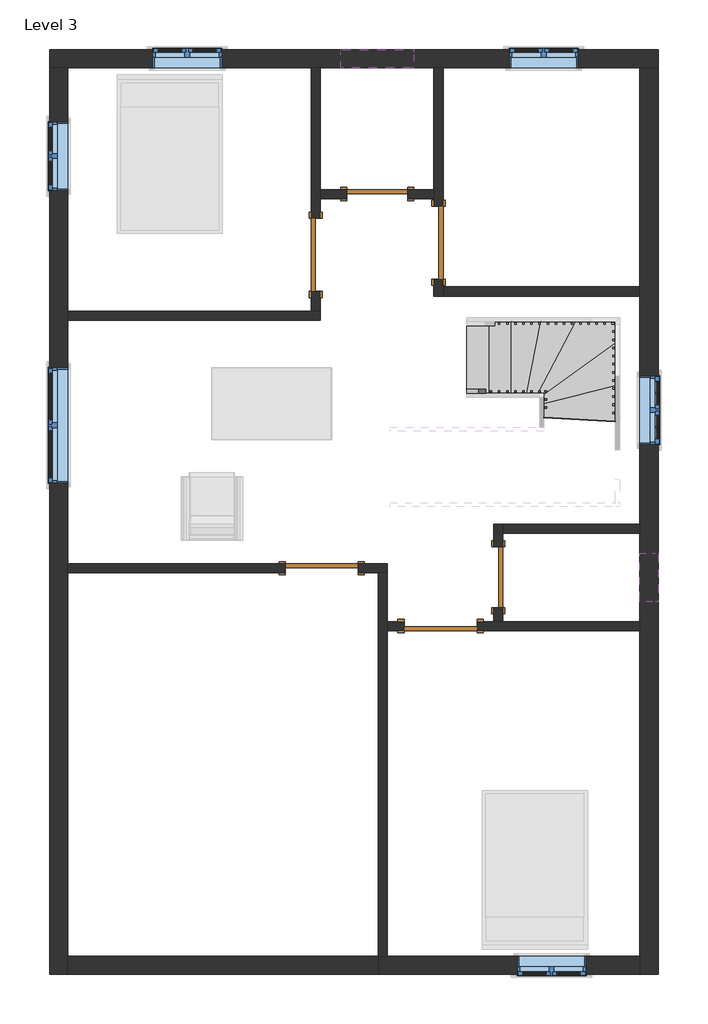
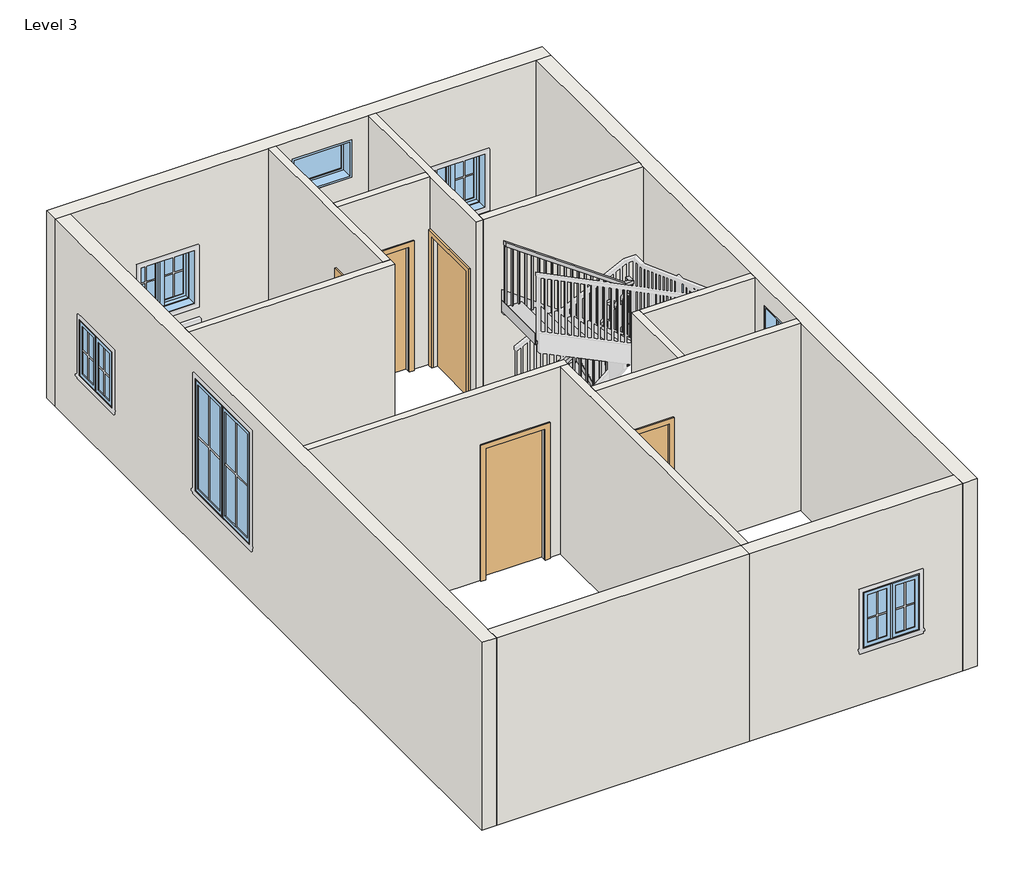
# One storey, part 1 of 2: 15 walls, 8 windows, 6 doors, 1 railing, 1 stair flight.
"""IFC4 building model written with IfcOpenShell, lengths in millimetres."""

from ifc_helpers import new_model, si_unit, frame, origin, place, context, project, spatial, polyline, outline, extrude, faceted_brep, transform, mapped, element, save
from components import door_d8f5dbb5, door_f2b275c1, door_e5f9f3c4, door_305aa2a5, stair_flight_546a6d32, window_80340324, window_bb95b1c9, window_339605e1, window_9ac97e1a

model = new_model("IFC4")

# Units and contexts
model_context = context("Model", 3, world=origin())
ifc_project = project(units=[si_unit("LENGTHUNIT", "METRE", prefix="MILLI")], contexts=[model_context])

# Site, building, storey
site = spatial("IfcSite", under=ifc_project)
building = spatial("IfcBuilding", under=site)
storey = spatial("IfcBuildingStorey", under=building, Name="Level 3", Elevation=3200.4)

# Doors
placement = place(None, origin())
door_shape = door_d8f5dbb5(model_context)
element("IfcDoor", 1, ObjectType="Single-Flush : 30\" x 80\"", at=placement, inside=storey, context=model_context, shape_type="MappedRepresentation", body=[
    mapped(door_shape, transform((-963.1415084, 4519.6435985, 3200.4), x_axis=(1.0, 0.0, 0.0), y_axis=(0.0, 1.0, 0.0), z_axis=(0.0, 0.0, 1.0))),
])
door_2_shape = door_f2b275c1(model_context)
element("IfcDoor", 2, ObjectType="Single-Flush : 30\" x 80\"", at=placement, inside=storey, context=model_context, shape_type="MappedRepresentation", body=[
    mapped(door_2_shape, transform((554.5084916, -280.9564015, 3200.4), x_axis=(0.0, 1.0, 0.0), y_axis=(-1.0, 0.0, 0.0), z_axis=(0.0, 0.0, 1.0))),
])
door_3_shape = door_e5f9f3c4(model_context)
element("IfcDoor", 3, ObjectType="Single-Flush : 36\" x 84\"", at=placement, inside=storey, context=model_context, shape_type="MappedRepresentation", body=[
    mapped(door_3_shape, transform((-194.7915084, 3910.0435985, 3200.4), x_axis=(0.0, -1.0, 0.0), y_axis=(1.0, 0.0, 0.0), z_axis=(0.0, 0.0, 1.0))),
])
element("IfcDoor", 4, ObjectType="Single-Flush : 36\" x 84\"", at=placement, inside=storey, context=model_context, shape_type="MappedRepresentation", body=[
    mapped(door_3_shape, transform((-1655.2915084, -166.6564015, 3200.4), x_axis=(1.0, 0.0, 0.0), y_axis=(0.0, 1.0, 0.0), z_axis=(0.0, 0.0, 1.0))),
])
element("IfcDoor", 5, ObjectType="Single-Flush : 36\" x 84\"", at=placement, inside=storey, context=model_context, shape_type="MappedRepresentation", body=[
    mapped(door_3_shape, transform((-169.3915084, -890.5564015, 3200.4), x_axis=(-1.0, 0.0, 0.0), y_axis=(0.0, -1.0, 0.0), z_axis=(0.0, 0.0, 1.0))),
])
door_4_shape = door_305aa2a5(model_context)
element("IfcDoor", 6, ObjectType="Single-Flush : 36\" x 84\"", at=placement, inside=storey, context=model_context, shape_type="MappedRepresentation", body=[
    mapped(door_4_shape, transform((-1731.4915084, 3757.6435985, 3200.4), x_axis=(0.0, -1.0, 0.0), y_axis=(1.0, 0.0, 0.0), z_axis=(0.0, 0.0, 1.0))),
])

# Railing
element("IfcRailing", 7, ObjectType="Handrail - Rectangular", at=placement, inside=storey, context=model_context, shape_type="SolidModel", body=[
    faceted_brep([(158.6923968, 2074.8935985, 4284.1333333), (158.6923968, 2074.8935985, 4220.4053174), (158.6923968, 2024.0935985, 4220.4053174), (158.6923968, 2024.0935985, 4284.1333333), (1047.1901835, 2074.8935985, 4957.132376), (1097.9901835, 2074.8935985, 4931.8831856), (1097.9901835, 2024.0935985, 4931.8831856), (1047.1901835, 2024.0935985, 4957.132376), (1047.1901835, 2074.8935985, 5211.4303182), (1097.9901835, 2074.8935985, 5160.6303182), (1097.9901835, 2024.0935985, 5160.6303182), (1047.1901835, 2024.0935985, 5211.4303182), (1174.1901835, 2074.8935985, 5211.4303182), (1174.1901835, 2074.8935985, 5160.6303182), (1123.3901835, 2024.0935985, 5160.6303182), (1123.3901835, 2024.0935985, 5211.4303182), (1174.1901835, 1947.8935985, 5211.4303182), (1174.1901835, 1922.7437783, 5160.6303182), (1123.3901835, 1922.7437783, 5160.6303182), (1123.3901835, 1947.8935985, 5211.4303182), (1174.1901835, 1627.4476133, 5631.73697), (1174.1901835, 1576.6476133, 5614.5805221), (1123.3901835, 1576.6476133, 5614.5805221), (1123.3901835, 1627.4476133, 5631.73697), (1174.1901835, 1627.4476133, 5852.9821577), (1174.1901835, 1576.6476133, 5802.1821577), (1123.3901835, 1576.6476133, 5802.1821577), (1123.3901835, 1627.4476133, 5852.9821577), (1174.1901835, 1500.4476133, 5852.9821577), (1174.1901835, 1500.4476133, 5802.1821577), (1123.3901835, 1551.2476133, 5802.1821577), (1123.3901835, 1551.2476133, 5852.9821577), (1047.1901835, 1500.4476133, 5852.9821577), (1030.9951821, 1500.4476133, 5802.1821577), (1030.9951821, 1551.2476133, 5802.1821577), (1047.1901835, 1551.2476133, 5852.9821577), (-798.3242294, 1500.4476133, 7162.8), (-798.3242294, 1551.2476133, 7162.8), (-798.3242294, 1551.2476133, 7100.5059138), (-798.3242294, 1500.4476133, 7100.5059138)], [[[0, 1, 2, 3]], [[1, 0, 4, 5]], [[2, 1, 5, 6]], [[3, 2, 6, 7]], [[0, 3, 7, 4]], [[5, 4, 8, 9]], [[6, 5, 9, 10]], [[7, 6, 10, 11]], [[4, 7, 11, 8]], [[9, 8, 12, 13]], [[10, 9, 13, 14]], [[11, 10, 14, 15]], [[8, 11, 15, 12]], [[13, 12, 16, 17]], [[14, 13, 17, 18]], [[15, 14, 18, 19]], [[12, 15, 19, 16]], [[17, 16, 20, 21]], [[18, 17, 21, 22]], [[19, 18, 22, 23]], [[16, 19, 23, 20]], [[21, 20, 24, 25]], [[22, 21, 25, 26]], [[23, 22, 26, 27]], [[20, 23, 27, 24]], [[25, 24, 28, 29]], [[26, 25, 29, 30]], [[27, 26, 30, 31]], [[24, 27, 31, 28]], [[29, 28, 32, 33]], [[30, 29, 33, 34]], [[31, 30, 34, 35]], [[28, 31, 35, 32]], [[36, 37, 38, 39]], [[33, 32, 36, 39]], [[34, 33, 39, 38]], [[35, 34, 38, 37]], [[32, 35, 37, 36]]]),
    extrude(outline(polyline([(7081.8830025, -772.0848165), (7095.4033683, -791.1348165), (6079.0666667, -791.1348165), (6079.0666667, -772.0848165), (7081.8830025, -772.0848165)])), frame((0.0, 1516.3226133, 0.0), z_axis=(0.0, 1.0, 0.0), x_axis=(0.0, 0.0, 1.0)), (0.0, 0.0, 1.0), 19.05),
    extrude(outline(polyline([(7009.7743851, -670.4848165), (7023.2947509, -689.5348165), (6079.0666667, -689.5348165), (6079.0666667, -670.4848165), (7009.7743851, -670.4848165)])), frame((0.0, 1516.3226133, 0.0), z_axis=(0.0, 1.0, 0.0), x_axis=(0.0, 0.0, 1.0)), (0.0, 0.0, 1.0), 19.05),
    extrude(outline(polyline([(6937.6657677, -568.8848165), (6951.1861334, -587.9348165), (6079.0666667, -587.9348165), (6079.0666667, -568.8848165), (6937.6657677, -568.8848165)])), frame((0.0, 1516.3226133, 0.0), z_axis=(0.0, 1.0, 0.0), x_axis=(0.0, 0.0, 1.0)), (0.0, 0.0, 1.0), 19.05),
    extrude(outline(polyline([(6865.5571502, -467.2848165), (6879.077516, -486.3348165), (5909.7333333, -486.3348165), (5909.7333333, -467.2848165), (6865.5571502, -467.2848165)])), frame((0.0, 1516.3226133, 0.0), z_axis=(0.0, 1.0, 0.0), x_axis=(0.0, 0.0, 1.0)), (0.0, 0.0, 1.0), 19.05),
    extrude(outline(polyline([(6793.4485328, -365.6848165), (6806.9688986, -384.7348165), (5909.7333333, -384.7348165), (5909.7333333, -365.6848165), (6793.4485328, -365.6848165)])), frame((0.0, 1516.3226133, 0.0), z_axis=(0.0, 1.0, 0.0), x_axis=(0.0, 0.0, 1.0)), (0.0, 0.0, 1.0), 19.05),
    extrude(outline(polyline([(6721.3399154, -264.0848165), (6734.8602811, -283.1348165), (5909.7333333, -283.1348165), (5909.7333333, -264.0848165), (6721.3399154, -264.0848165)])), frame((0.0, 1516.3226133, 0.0), z_axis=(0.0, 1.0, 0.0), x_axis=(0.0, 0.0, 1.0)), (0.0, 0.0, 1.0), 19.05),
    extrude(outline(polyline([(6649.2312979, -162.4848165), (6662.7516637, -181.5348165), (5740.4, -181.5348165), (5740.4, -162.4848165), (6649.2312979, -162.4848165)])), frame((0.0, 1516.3226133, 0.0), z_axis=(0.0, 1.0, 0.0), x_axis=(0.0, 0.0, 1.0)), (0.0, 0.0, 1.0), 19.05),
    extrude(outline(polyline([(6577.1226805, -60.8848165), (6590.6430462, -79.9348165), (5740.4, -79.9348165), (5740.4, -60.8848165), (6577.1226805, -60.8848165)])), frame((0.0, 1516.3226133, 0.0), z_axis=(0.0, 1.0, 0.0), x_axis=(0.0, 0.0, 1.0)), (0.0, 0.0, 1.0), 19.05),
    extrude(outline(polyline([(6505.014063, 40.7151835), (6518.5344288, 21.6651835), (5571.0666667, 21.6651835), (5571.0666667, 40.7151835), (6505.014063, 40.7151835)])), frame((0.0, 1516.3226133, 0.0), z_axis=(0.0, 1.0, 0.0), x_axis=(0.0, 0.0, 1.0)), (0.0, 0.0, 1.0), 19.05),
    extrude(outline(polyline([(6432.9054456, 142.3151835), (6446.4258114, 123.2651835), (5571.0666667, 123.2651835), (5571.0666667, 142.3151835), (6432.9054456, 142.3151835)])), frame((0.0, 1516.3226133, 0.0), z_axis=(0.0, 1.0, 0.0), x_axis=(0.0, 0.0, 1.0)), (0.0, 0.0, 1.0), 19.05),
    extrude(outline(polyline([(6360.7968282, 243.9151835), (6374.3171939, 224.8651835), (5571.0666667, 224.8651835), (5571.0666667, 243.9151835), (6360.7968282, 243.9151835)])), frame((0.0, 1516.3226133, 0.0), z_axis=(0.0, 1.0, 0.0), x_axis=(0.0, 0.0, 1.0)), (0.0, 0.0, 1.0), 19.05),
    extrude(outline(polyline([(6288.6882107, 345.5151835), (6302.2085765, 326.4651835), (5401.7333333, 326.4651835), (5401.7333333, 345.5151835), (6288.6882107, 345.5151835)])), frame((0.0, 1516.3226133, 0.0), z_axis=(0.0, 1.0, 0.0), x_axis=(0.0, 0.0, 1.0)), (0.0, 0.0, 1.0), 19.05),
    extrude(outline(polyline([(6216.5795933, 447.1151835), (6230.0999591, 428.0651835), (5401.7333333, 428.0651835), (5401.7333333, 447.1151835), (6216.5795933, 447.1151835)])), frame((0.0, 1516.3226133, 0.0), z_axis=(0.0, 1.0, 0.0), x_axis=(0.0, 0.0, 1.0)), (0.0, 0.0, 1.0), 19.05),
    extrude(outline(polyline([(6144.4709758, 548.7151835), (6157.9913416, 529.6651835), (5232.4, 529.6651835), (5232.4, 548.7151835), (6144.4709758, 548.7151835)])), frame((0.0, 1516.3226133, 0.0), z_axis=(0.0, 1.0, 0.0), x_axis=(0.0, 0.0, 1.0)), (0.0, 0.0, 1.0), 19.05),
    extrude(outline(polyline([(6072.3623584, 650.3151835), (6085.8827242, 631.2651835), (5232.4, 631.2651835), (5232.4, 650.3151835), (6072.3623584, 650.3151835)])), frame((0.0, 1516.3226133, 0.0), z_axis=(0.0, 1.0, 0.0), x_axis=(0.0, 0.0, 1.0)), (0.0, 0.0, 1.0), 19.05),
    extrude(outline(polyline([(6000.253741, 751.9151835), (6013.7741067, 732.8651835), (5232.4, 732.8651835), (5232.4, 751.9151835), (6000.253741, 751.9151835)])), frame((0.0, 1516.3226133, 0.0), z_axis=(0.0, 1.0, 0.0), x_axis=(0.0, 0.0, 1.0)), (0.0, 0.0, 1.0), 19.05),
    extrude(outline(polyline([(5928.1451235, 853.5151835), (5941.6654893, 834.4651835), (5063.0666667, 834.4651835), (5063.0666667, 853.5151835), (5928.1451235, 853.5151835)])), frame((0.0, 1516.3226133, 0.0), z_axis=(0.0, 1.0, 0.0), x_axis=(0.0, 0.0, 1.0)), (0.0, 0.0, 1.0), 19.05),
    extrude(outline(polyline([(5856.0365061, 955.1151835), (5869.5568719, 936.0651835), (5063.0666667, 936.0651835), (5063.0666667, 955.1151835), (5856.0365061, 955.1151835)])), frame((0.0, 1516.3226133, 0.0), z_axis=(0.0, 1.0, 0.0), x_axis=(0.0, 0.0, 1.0)), (0.0, 0.0, 1.0), 19.05),
    extrude(outline(polyline([(5783.9278887, 1056.7151835), (5797.4482544, 1037.6651835), (4893.7333333, 1037.6651835), (4893.7333333, 1056.7151835), (5783.9278887, 1056.7151835)])), frame((0.0, 1516.3226133, 0.0), z_axis=(0.0, 1.0, 0.0), x_axis=(0.0, 0.0, 1.0)), (0.0, 0.0, 1.0), 19.05),
    extrude(outline(polyline([(1139.2651835, 1551.0185985), (1158.3151835, 1551.0185985), (1158.3151835, 1531.9685985), (1139.2651835, 1531.9685985), (1139.2651835, 1551.0185985)])), frame((0.0, 0.0, 4724.4), z_axis=(0.0, 0.0, 1.0), x_axis=(1.0, 0.0, 0.0)), (0.0, 0.0, 1.0), 1077.7821578),
    extrude(outline(polyline([(1633.5685985, 5539.9212353), (1652.6185985, 5514.9346787), (1652.6185985, 4555.0666667), (1633.5685985, 4555.0666667), (1633.5685985, 5539.9212353)])), frame((1139.2651835, 0.0, 0.0), z_axis=(1.0, 0.0, 0.0), x_axis=(0.0, 1.0, 0.0)), (0.0, 0.0, 1.0), 19.05),
    extrude(outline(polyline([(1735.1685985, 5406.6596006), (1754.2185985, 5381.673044), (1754.2185985, 4555.0666667), (1735.1685985, 4555.0666667), (1735.1685985, 5406.6596006)])), frame((1139.2651835, 0.0, 0.0), z_axis=(1.0, 0.0, 0.0), x_axis=(0.0, 1.0, 0.0)), (0.0, 0.0, 1.0), 19.05),
    extrude(outline(polyline([(1836.7685985, 5273.3979659), (1855.8185985, 5248.4114093), (1855.8185985, 4385.7333333), (1836.7685985, 4385.7333333), (1836.7685985, 5273.3979659)])), frame((1139.2651835, 0.0, 0.0), z_axis=(1.0, 0.0, 0.0), x_axis=(0.0, 1.0, 0.0)), (0.0, 0.0, 1.0), 19.05),
    extrude(outline(polyline([(1938.3685985, 5140.1363312), (1957.4185985, 5115.1497746), (1957.4185985, 4216.4), (1938.3685985, 4216.4), (1938.3685985, 5140.1363312)])), frame((1139.2651835, 0.0, 0.0), z_axis=(1.0, 0.0, 0.0), x_axis=(0.0, 1.0, 0.0)), (0.0, 0.0, 1.0), 19.05),
    extrude(outline(polyline([(1063.5673968, 2039.9685985), (1063.5673968, 2059.0185985), (1082.6173968, 2059.0185985), (1082.6173968, 2039.9685985), (1063.5673968, 2039.9685985)])), frame((0.0, 0.0, 4047.0666667), z_axis=(0.0, 0.0, 1.0), x_axis=(1.0, 0.0, 0.0)), (0.0, 0.0, 1.0), 1113.5636515),
    extrude(outline(polyline([(4843.2813066, 981.0173968), (4828.851747, 961.9673968), (3877.7333333, 961.9673968), (3877.7333333, 981.0173968), (4843.2813066, 981.0173968)])), frame((0.0, 2039.9685985, 0.0), z_axis=(0.0, 1.0, 0.0), x_axis=(0.0, 0.0, 1.0)), (0.0, 0.0, 1.0), 19.05),
    extrude(outline(polyline([(4766.3236554, 879.4173968), (4751.8940958, 860.3673968), (3708.4, 860.3673968), (3708.4, 879.4173968), (4766.3236554, 879.4173968)])), frame((0.0, 2039.9685985, 0.0), z_axis=(0.0, 1.0, 0.0), x_axis=(0.0, 0.0, 1.0)), (0.0, 0.0, 1.0), 19.05),
    extrude(outline(polyline([(4689.3660042, 777.8173968), (4674.9364446, 758.7673968), (3708.4, 758.7673968), (3708.4, 777.8173968), (4689.3660042, 777.8173968)])), frame((0.0, 2039.9685985, 0.0), z_axis=(0.0, 1.0, 0.0), x_axis=(0.0, 0.0, 1.0)), (0.0, 0.0, 1.0), 19.05),
    extrude(outline(polyline([(4612.408353, 676.2173968), (4597.9787934, 657.1673968), (3539.0666667, 657.1673968), (3539.0666667, 676.2173968), (4612.408353, 676.2173968)])), frame((0.0, 2039.9685985, 0.0), z_axis=(0.0, 1.0, 0.0), x_axis=(0.0, 0.0, 1.0)), (0.0, 0.0, 1.0), 19.05),
    extrude(outline(polyline([(4535.4507019, 574.6173968), (4521.0211423, 555.5673968), (3539.0666667, 555.5673968), (3539.0666667, 574.6173968), (4535.4507019, 574.6173968)])), frame((0.0, 2039.9685985, 0.0), z_axis=(0.0, 1.0, 0.0), x_axis=(0.0, 0.0, 1.0)), (0.0, 0.0, 1.0), 19.05),
    extrude(outline(polyline([(4458.4930507, 473.0173968), (4444.0634911, 453.9673968), (3539.0666667, 453.9673968), (3539.0666667, 473.0173968), (4458.4930507, 473.0173968)])), frame((0.0, 2039.9685985, 0.0), z_axis=(0.0, 1.0, 0.0), x_axis=(0.0, 0.0, 1.0)), (0.0, 0.0, 1.0), 19.05),
    extrude(outline(polyline([(4381.5353995, 371.4173968), (4367.1058399, 352.3673968), (3369.7333333, 352.3673968), (3369.7333333, 371.4173968), (4381.5353995, 371.4173968)])), frame((0.0, 2039.9685985, 0.0), z_axis=(0.0, 1.0, 0.0), x_axis=(0.0, 0.0, 1.0)), (0.0, 0.0, 1.0), 19.05),
    extrude(outline(polyline([(4304.5777483, 269.8173968), (4290.1481887, 250.7673968), (3369.7333333, 250.7673968), (3369.7333333, 269.8173968), (4304.5777483, 269.8173968)])), frame((0.0, 2039.9685985, 0.0), z_axis=(0.0, 1.0, 0.0), x_axis=(0.0, 0.0, 1.0)), (0.0, 0.0, 1.0), 19.05),
    extrude(outline(polyline([(1139.2651835, 1535.3726133), (1158.3151835, 1535.3726133), (1158.3151835, 1516.3226133), (1139.2651835, 1516.3226133), (1139.2651835, 1535.3726133)])), frame((0.0, 0.0, 4724.4), z_axis=(0.0, 0.0, 1.0), x_axis=(1.0, 0.0, 0.0)), (0.0, 0.0, 1.0), 1077.7821578),
    extrude(outline(polyline([(1139.2651835, 2039.9685985), (1139.2651835, 2059.0185985), (1158.3151835, 2059.0185985), (1158.3151835, 2039.9685985), (1139.2651835, 2039.9685985)])), frame((0.0, 0.0, 4047.0666667), z_axis=(0.0, 0.0, 1.0), x_axis=(1.0, 0.0, 0.0)), (0.0, 0.0, 1.0), 1113.5636515),
    extrude(outline(polyline([(7086.985548, -779.2742294), (7100.5059138, -798.3242294), (6079.0666667, -798.3242294), (6079.0666667, -779.2742294), (7086.985548, -779.2742294)])), frame((0.0, 1516.3226133, 0.0), z_axis=(0.0, 1.0, 0.0), x_axis=(0.0, 0.0, 1.0)), (0.0, 0.0, 1.0), 19.05),
    extrude(outline(polyline([(4234.834877, 177.7423968), (4220.4053174, 158.6923968), (3369.7333333, 158.6923968), (3369.7333333, 177.7423968), (4234.834877, 177.7423968)])), frame((0.0, 2039.9685985, 0.0), z_axis=(0.0, 1.0, 0.0), x_axis=(0.0, 0.0, 1.0)), (0.0, 0.0, 1.0), 19.05),
])

# Stair flight
stair_flight_shape = stair_flight_546a6d32(model_context)
element("IfcStairFlight", 8, ObjectType="2\" Tread 1\" Nosing 1/4\" Riser", at=placement, inside=storey, context=model_context, shape_type="MappedRepresentation", body=[
    mapped(stair_flight_shape, transform((0.0, 0.0, 0.0), x_axis=(1.0, 0.0, 0.0), y_axis=(0.0, 1.0, 0.0), z_axis=(0.0, 0.0, 1.0))),
])

# Walls
element("IfcWall", 9, ObjectType="WALL4.5\"", at=placement, inside=storey, context=model_context, shape_type="Brep", body=[
    faceted_brep([(-4836.6415084, 2938.4935985, 3200.4), (-1674.3415084, 2938.4935985, 3200.4), (-1674.3415084, 2938.4935985, 6248.4), (-4836.6415084, 2938.4935985, 6248.4), (-4836.6415084, 3052.7935985, 3200.4), (-4836.6415084, 3052.7935985, 6248.4), (-1788.6415084, 3052.7935985, 6248.4), (-1674.3415084, 3052.7935985, 6248.4), (-1674.3415084, 3052.7935985, 3200.4), (-1788.6415084, 3052.7935985, 3200.4)], [[[0, 1, 2, 3]], [[4, 5, 6, 7, 8, 9]], [[1, 0, 4, 9, 8]], [[0, 3, 5, 4]], [[2, 1, 8, 7]], [[3, 2, 7, 6, 5]]]),
])
element("IfcWall", 10, ObjectType="WALL4.5\"", at=placement, inside=storey, context=model_context, shape_type="Brep", body=[
    faceted_brep([(-1674.3415084, 3052.7935985, 3200.4), (-1674.3415084, 3300.4435985, 3200.4), (-1674.3415084, 3300.4435985, 5334.0), (-1674.3415084, 4214.8435985, 5334.0), (-1674.3415084, 4214.8435985, 3200.4), (-1674.3415084, 4462.4935985, 3200.4), (-1674.3415084, 4576.7935985, 3200.4), (-1674.3415084, 6100.7935985, 3200.4), (-1674.3415084, 6100.7935985, 6248.4), (-1674.3415084, 4576.7935985, 6248.4), (-1674.3415084, 4462.4935985, 6248.4), (-1674.3415084, 3052.7935985, 6248.4), (-1788.6415084, 3300.4435985, 5334.0), (-1788.6415084, 3300.4435985, 3200.4), (-1788.6415084, 3052.7935985, 3200.4), (-1788.6415084, 3052.7935985, 6248.4), (-1788.6415084, 6100.7935985, 6248.4), (-1788.6415084, 6100.7935985, 3200.4), (-1788.6415084, 4214.8435985, 3200.4), (-1788.6415084, 4214.8435985, 5334.0)], [[[0, 1, 2, 3, 4, 5, 6, 7, 8, 9, 10, 11]], [[12, 13, 14, 15, 16, 17, 18, 19]], [[18, 17, 7, 6, 5, 4]], [[14, 13, 1, 0]], [[0, 11, 15, 14]], [[8, 7, 17, 16]], [[2, 1, 13, 12]], [[3, 2, 12, 19]], [[4, 3, 19, 18]], [[11, 10, 9, 8, 16, 15]]]),
])
element("IfcWall", 11, ObjectType="WALL4.5\"", at=placement, inside=storey, context=model_context, shape_type="SweptSolid", body=[
    extrude(outline(polyline([(5232.4, -582.1415084), (3200.4, -582.1415084), (3200.4, -251.9415084), (6248.4, -251.9415084), (6248.4, -1674.3415084), (3200.4, -1674.3415084), (3200.4, -1344.1415084), (5232.4, -1344.1415084), (5232.4, -582.1415084)])), frame((0.0, 4462.4935985, 0.0), z_axis=(0.0, 1.0, 0.0), x_axis=(0.0, 0.0, 1.0)), (0.0, 0.0, 1.0), 114.3),
])
element("IfcWall", 12, ObjectType="WALL4.5\"", at=placement, inside=storey, context=model_context, shape_type="Brep", body=[
    faceted_brep([(-251.9415084, 3452.8435985, 5334.0), (-251.9415084, 3452.8435985, 3200.4), (-251.9415084, 3243.2935985, 3200.4), (-251.9415084, 3243.2935985, 6248.4), (-251.9415084, 4462.4935985, 6248.4), (-251.9415084, 4576.7935985, 6248.4), (-251.9415084, 6100.7935985, 6248.4), (-251.9415084, 6100.7935985, 3200.4), (-251.9415084, 4576.7935985, 3200.4), (-251.9415084, 4462.4935985, 3200.4), (-251.9415084, 4367.2435985, 3200.4), (-251.9415084, 4367.2435985, 5334.0), (-137.6415084, 3243.2935985, 3200.4), (-137.6415084, 3357.5935985, 3200.4), (-137.6415084, 3452.8435985, 3200.4), (-137.6415084, 3452.8435985, 5334.0), (-137.6415084, 4367.2435985, 5334.0), (-137.6415084, 4367.2435985, 3200.4), (-137.6415084, 6100.7935985, 3200.4), (-137.6415084, 6100.7935985, 6248.4), (-137.6415084, 3357.5935985, 6248.4), (-137.6415084, 3243.2935985, 6248.4)], [[[0, 1, 2, 3, 4, 5, 6, 7, 8, 9, 10, 11]], [[12, 13, 14, 15, 16, 17, 18, 19, 20, 21]], [[2, 1, 14, 13, 12]], [[10, 9, 8, 7, 18, 17]], [[7, 6, 19, 18]], [[3, 2, 12, 21]], [[15, 14, 1, 0]], [[16, 15, 0, 11]], [[17, 16, 11, 10]], [[6, 5, 4, 3, 21, 20, 19]]]),
])
element("IfcWall", 13, ObjectType="WALL4.5\"", at=placement, inside=storey, context=model_context, shape_type="SweptSolid", body=[
    extrude(outline(polyline([(2326.1584916, 3243.2935985), (-137.6415084, 3243.2935985), (-137.6415084, 3357.5935985), (2326.1584916, 3357.5935985), (2326.1584916, 3243.2935985)])), frame((0.0, 0.0, 3200.4), z_axis=(0.0, 0.0, 1.0), x_axis=(1.0, 0.0, 0.0)), (0.0, 0.0, 1.0), 3048.0),
])
element("IfcWall", 14, ObjectType="WALL4.5\"", at=placement, inside=storey, context=model_context, shape_type="Brep", body=[
    faceted_brep([(-1198.0915084, -223.8064015, 5334.0), (-1198.0915084, -223.8064015, 3200.4), (-950.4415084, -223.8064015, 3200.4), (-836.1415084, -223.8064015, 3200.4), (-836.1415084, -223.8064015, 6248.4), (-950.4415084, -223.8064015, 6248.4), (-4836.6415084, -223.8064015, 6248.4), (-4836.6415084, -223.8064015, 3200.4), (-2112.4915084, -223.8064015, 3200.4), (-2112.4915084, -223.8064015, 5334.0), (-836.1415084, -109.5064015, 3200.4), (-1198.0915084, -109.5064015, 3200.4), (-1198.0915084, -109.5064015, 5334.0), (-2112.4915084, -109.5064015, 5334.0), (-2112.4915084, -109.5064015, 3200.4), (-4836.6415084, -109.5064015, 3200.4), (-4836.6415084, -109.5064015, 6248.4), (-836.1415084, -109.5064015, 6248.4)], [[[0, 1, 2, 3, 4, 5, 6, 7, 8, 9]], [[10, 11, 12, 13, 14, 15, 16, 17]], [[8, 7, 15, 14]], [[3, 2, 1, 11, 10]], [[7, 6, 16, 15]], [[4, 3, 10, 17]], [[12, 11, 1, 0]], [[13, 12, 0, 9]], [[14, 13, 9, 8]], [[6, 5, 4, 17, 16]]]),
])
element("IfcWall", 15, ObjectType="WALL4.5\"", at=placement, inside=storey, context=model_context, shape_type="Brep", body=[
    faceted_brep([(-950.4415084, -223.8064015, 3200.4), (-950.4415084, -5024.4064015, 3200.4), (-950.4415084, -5024.4064015, 6248.4), (-950.4415084, -223.8064015, 6248.4), (-836.1415084, -223.8064015, 3200.4), (-836.1415084, -223.8064015, 6248.4), (-836.1415084, -833.4064015, 6248.4), (-836.1415084, -947.7064015, 6248.4), (-836.1415084, -5024.4064015, 6248.4), (-836.1415084, -5024.4064015, 3200.4), (-836.1415084, -947.7064015, 3200.4), (-836.1415084, -833.4064015, 3200.4)], [[[0, 1, 2, 3]], [[4, 5, 6, 7, 8, 9, 10, 11]], [[2, 1, 9, 8]], [[0, 3, 5, 4]], [[1, 0, 4, 11, 10, 9]], [[3, 2, 8, 7, 6, 5]]]),
])
element("IfcWall", 16, ObjectType="WALL4.5\"", at=placement, inside=storey, context=model_context, shape_type="Brep", body=[
    faceted_brep([(-836.1415084, -947.7064015, 3200.4), (-626.5915084, -947.7064015, 3200.4), (-626.5915084, -947.7064015, 5334.0), (287.8084916, -947.7064015, 5334.0), (287.8084916, -947.7064015, 3200.4), (2326.1584916, -947.7064015, 3200.4), (2326.1584916, -947.7064015, 6248.4), (-836.1415084, -947.7064015, 6248.4), (-626.5915084, -833.4064015, 5334.0), (-626.5915084, -833.4064015, 3200.4), (-836.1415084, -833.4064015, 3200.4), (-836.1415084, -833.4064015, 6248.4), (497.3584916, -833.4064015, 6248.4), (611.6584916, -833.4064015, 6248.4), (2326.1584916, -833.4064015, 6248.4), (2326.1584916, -833.4064015, 3200.4), (611.6584916, -833.4064015, 3200.4), (497.3584916, -833.4064015, 3200.4), (287.8084916, -833.4064015, 3200.4), (287.8084916, -833.4064015, 5334.0)], [[[0, 1, 2, 3, 4, 5, 6, 7]], [[8, 9, 10, 11, 12, 13, 14, 15, 16, 17, 18, 19]], [[10, 9, 1, 0]], [[18, 17, 16, 15, 5, 4]], [[6, 5, 15, 14]], [[0, 7, 11, 10]], [[2, 1, 9, 8]], [[3, 2, 8, 19]], [[4, 3, 19, 18]], [[7, 6, 14, 13, 12, 11]]]),
])
element("IfcWall", 17, ObjectType="WALL4.5\"", at=placement, inside=storey, context=model_context, shape_type="Brep", body=[
    faceted_brep([(611.6584916, 100.0435985, 5232.4), (611.6584916, 100.0435985, 3200.4), (611.6584916, 271.4935985, 3200.4), (611.6584916, 385.7935985, 3200.4), (611.6584916, 385.7935985, 6248.4), (611.6584916, 271.4935985, 6248.4), (611.6584916, -833.4064015, 6248.4), (611.6584916, -833.4064015, 3200.4), (611.6584916, -661.9564015, 3200.4), (611.6584916, -661.9564015, 5232.4), (497.3584916, 385.7935985, 3200.4), (497.3584916, 100.0435985, 3200.4), (497.3584916, 100.0435985, 5232.4), (497.3584916, -661.9564015, 5232.4), (497.3584916, -661.9564015, 3200.4), (497.3584916, -833.4064015, 3200.4), (497.3584916, -833.4064015, 6248.4), (497.3584916, 385.7935985, 6248.4)], [[[0, 1, 2, 3, 4, 5, 6, 7, 8, 9]], [[10, 11, 12, 13, 14, 15, 16, 17]], [[8, 7, 15, 14]], [[3, 2, 1, 11, 10]], [[7, 6, 16, 15]], [[4, 3, 10, 17]], [[12, 11, 1, 0]], [[13, 12, 0, 9]], [[14, 13, 9, 8]], [[6, 5, 4, 17, 16]]]),
])
element("IfcWall", 18, ObjectType="WALL4.5\"", at=placement, inside=storey, context=model_context, shape_type="SweptSolid", body=[
    extrude(outline(polyline([(2326.1584916, 271.4935985), (611.6584916, 271.4935985), (611.6584916, 385.7935985), (2326.1584916, 385.7935985), (2326.1584916, 271.4935985)])), frame((0.0, 0.0, 3200.4), z_axis=(0.0, 0.0, 1.0), x_axis=(1.0, 0.0, 0.0)), (0.0, 0.0, 1.0), 3048.0),
])
element("IfcWall", 19, ObjectType="WALL9\"", at=placement, inside=storey, context=model_context, shape_type="Brep", body=[
    faceted_brep([(-5065.2415084, 6100.7935985, 3200.4), (-4836.6415084, 6100.7935985, 3200.4), (-1788.6415084, 6100.7935985, 3200.4), (-1674.3415084, 6100.7935985, 3200.4), (-251.9415084, 6100.7935985, 3200.4), (-137.6415084, 6100.7935985, 3200.4), (2326.1584916, 6100.7935985, 3200.4), (2554.7584916, 6100.7935985, 3200.4), (2554.7584916, 6100.7935985, 6248.4), (2326.1584916, 6100.7935985, 6248.4), (-137.6415084, 6100.7935985, 6248.4), (-251.9415084, 6100.7935985, 6248.4), (-1674.3415084, 6100.7935985, 6248.4), (-1788.6415084, 6100.7935985, 6248.4), (-4836.6415084, 6100.7935985, 6248.4), (-5065.2415084, 6100.7935985, 6248.4), (-505.9415084, 6100.7935985, 5943.6), (-505.9415084, 6100.7935985, 5334.0), (-1420.3415084, 6100.7935985, 5334.0), (-1420.3415084, 6100.7935985, 5943.6), (-2909.4165084, 6100.7935985, 5029.2), (-2909.4165084, 6100.7935985, 4114.8), (-3773.0165084, 6100.7935985, 4114.8), (-3773.0165084, 6100.7935985, 5029.2), (1554.6334916, 6100.7935985, 5029.2), (1554.6334916, 6100.7935985, 4114.8), (691.0334916, 6100.7935985, 4114.8), (691.0334916, 6100.7935985, 5029.2), (-5065.2415084, 6329.3935985, 3200.4), (-5065.2415084, 6329.3935985, 6248.4), (2554.7584916, 6329.3935985, 6248.4), (2554.7584916, 6329.3935985, 3200.4), (-505.9415084, 6329.3935985, 5943.6), (-1420.3415084, 6329.3935985, 5943.6), (-1420.3415084, 6329.3935985, 5334.0), (-505.9415084, 6329.3935985, 5334.0), (-2909.4165084, 6329.3935985, 5029.2), (-3773.0165084, 6329.3935985, 5029.2), (-3773.0165084, 6329.3935985, 4114.8), (-2909.4165084, 6329.3935985, 4114.8), (1554.6334916, 6329.3935985, 5029.2), (691.0334916, 6329.3935985, 5029.2), (691.0334916, 6329.3935985, 4114.8), (1554.6334916, 6329.3935985, 4114.8)], [[[0, 1, 2, 3, 4, 5, 6, 7, 8, 9, 10, 11, 12, 13, 14, 15], [16, 17, 18, 19], [20, 21, 22, 23], [24, 25, 26, 27]], [[28, 29, 30, 31], [32, 33, 34, 35], [36, 37, 38, 39], [40, 41, 42, 43]], [[7, 6, 5, 4, 3, 2, 1, 0, 28, 31]], [[8, 7, 31, 30]], [[0, 15, 29, 28]], [[17, 16, 32, 35]], [[18, 17, 35, 34]], [[19, 18, 34, 33]], [[16, 19, 33, 32]], [[21, 20, 36, 39]], [[22, 21, 39, 38]], [[23, 22, 38, 37]], [[20, 23, 37, 36]], [[25, 24, 40, 43]], [[26, 25, 43, 42]], [[27, 26, 42, 41]], [[24, 27, 41, 40]], [[15, 14, 13, 12, 11, 10, 9, 8, 30, 29]]]),
])
element("IfcWall", 20, ObjectType="WALL9\"", at=placement, inside=storey, context=model_context, shape_type="Brep", body=[
    faceted_brep([(2326.1584916, 6100.7935985, 3200.4), (2326.1584916, 3357.5935985, 3200.4), (2326.1584916, 3243.2935985, 3200.4), (2326.1584916, 385.7935985, 3200.4), (2326.1584916, 271.4935985, 3200.4), (2326.1584916, -833.4064015, 3200.4), (2326.1584916, -947.7064015, 3200.4), (2326.1584916, -5024.4064015, 3200.4), (2326.1584916, -5253.0064015, 3200.4), (2326.1584916, -5253.0064015, 6248.4), (2326.1584916, -5024.4064015, 6248.4), (2326.1584916, -947.7064015, 6248.4), (2326.1584916, -833.4064015, 6248.4), (2326.1584916, 271.4935985, 6248.4), (2326.1584916, 385.7935985, 6248.4), (2326.1584916, 3243.2935985, 6248.4), (2326.1584916, 3357.5935985, 6248.4), (2326.1584916, 6100.7935985, 6248.4), (2326.1584916, -585.7564015, 5943.6), (2326.1584916, -585.7564015, 5334.0), (2326.1584916, 23.8435985, 5334.0), (2326.1584916, 23.8435985, 5943.6), (2326.1584916, 1382.7435985, 5029.2), (2326.1584916, 1382.7435985, 4114.8), (2326.1584916, 2246.3435985, 4114.8), (2326.1584916, 2246.3435985, 5029.2), (2554.7584916, 6100.7935985, 3200.4), (2554.7584916, 6100.7935985, 6248.4), (2554.7584916, -5253.0064015, 6248.4), (2554.7584916, -5253.0064015, 3200.4), (2554.7584916, -585.7564015, 5943.6), (2554.7584916, 23.8435985, 5943.6), (2554.7584916, 23.8435985, 5334.0), (2554.7584916, -585.7564015, 5334.0), (2554.7584916, 1382.7435985, 5029.2), (2554.7584916, 2246.3435985, 5029.2), (2554.7584916, 2246.3435985, 4114.8), (2554.7584916, 1382.7435985, 4114.8)], [[[0, 1, 2, 3, 4, 5, 6, 7, 8, 9, 10, 11, 12, 13, 14, 15, 16, 17], [18, 19, 20, 21], [22, 23, 24, 25]], [[26, 27, 28, 29], [30, 31, 32, 33], [34, 35, 36, 37]], [[8, 7, 6, 5, 4, 3, 2, 1, 0, 26, 29]], [[0, 17, 27, 26]], [[9, 8, 29, 28]], [[19, 18, 30, 33]], [[20, 19, 33, 32]], [[21, 20, 32, 31]], [[18, 21, 31, 30]], [[23, 22, 34, 37]], [[24, 23, 37, 36]], [[25, 24, 36, 35]], [[22, 25, 35, 34]], [[17, 16, 15, 14, 13, 12, 11, 10, 9, 28, 27]]]),
])
element("IfcWall", 21, ObjectType="WALL9\"", at=placement, inside=storey, context=model_context, shape_type="Brep", body=[
    faceted_brep([(2326.1584916, -5024.4064015, 3200.4), (-836.1415084, -5024.4064015, 3200.4), (-950.4415084, -5024.4064015, 3200.4), (-950.4415084, -5024.4064015, 6248.4), (-836.1415084, -5024.4064015, 6248.4), (2326.1584916, -5024.4064015, 6248.4), (789.4584916, -5024.4064015, 5029.2), (789.4584916, -5024.4064015, 4114.8), (1653.0584916, -5024.4064015, 4114.8), (1653.0584916, -5024.4064015, 5029.2), (2326.1584916, -5253.0064015, 3200.4), (2326.1584916, -5253.0064015, 6248.4), (-950.4415084, -5253.0064015, 6248.4), (-950.4415084, -5253.0064015, 3200.4), (789.4584916, -5253.0064015, 5029.2), (1653.0584916, -5253.0064015, 5029.2), (1653.0584916, -5253.0064015, 4114.8), (789.4584916, -5253.0064015, 4114.8)], [[[0, 1, 2, 3, 4, 5], [6, 7, 8, 9]], [[10, 11, 12, 13], [14, 15, 16, 17]], [[2, 1, 0, 10, 13]], [[0, 5, 11, 10]], [[3, 2, 13, 12]], [[7, 6, 14, 17]], [[8, 7, 17, 16]], [[9, 8, 16, 15]], [[6, 9, 15, 14]], [[5, 4, 3, 12, 11]]]),
])
element("IfcWall", 22, ObjectType="WALL9\"", at=placement, inside=storey, context=model_context, shape_type="Brep", body=[
    faceted_brep([(-5065.2415084, 6100.7935985, 3200.4), (-5065.2415084, -5253.0064015, 3200.4), (-5065.2415084, -5253.0064015, 6248.4), (-5065.2415084, 6100.7935985, 6248.4), (-5065.2415084, 2347.9435985, 5943.6), (-5065.2415084, 900.1435985, 5943.6), (-5065.2415084, 900.1435985, 4114.8), (-5065.2415084, 2347.9435985, 4114.8), (-5065.2415084, 5427.6935985, 5029.2), (-5065.2415084, 4564.0935985, 5029.2), (-5065.2415084, 4564.0935985, 4114.8), (-5065.2415084, 5427.6935985, 4114.8), (-4836.6415084, 6100.7935985, 3200.4), (-4836.6415084, 6100.7935985, 6248.4), (-4836.6415084, 3052.7935985, 6248.4), (-4836.6415084, 2938.4935985, 6248.4), (-4836.6415084, -109.5064015, 6248.4), (-4836.6415084, -223.8064015, 6248.4), (-4836.6415084, -5024.4064015, 6248.4), (-4836.6415084, -5253.0064015, 6248.4), (-4836.6415084, -5253.0064015, 3200.4), (-4836.6415084, -5024.4064015, 3200.4), (-4836.6415084, -223.8064015, 3200.4), (-4836.6415084, -109.5064015, 3200.4), (-4836.6415084, 2938.4935985, 3200.4), (-4836.6415084, 3052.7935985, 3200.4), (-4836.6415084, 2347.9435985, 5943.6), (-4836.6415084, 2347.9435985, 4114.8), (-4836.6415084, 900.1435985, 4114.8), (-4836.6415084, 900.1435985, 5943.6), (-4836.6415084, 5427.6935985, 5029.2), (-4836.6415084, 5427.6935985, 4114.8), (-4836.6415084, 4564.0935985, 4114.8), (-4836.6415084, 4564.0935985, 5029.2)], [[[0, 1, 2, 3], [4, 5, 6, 7], [8, 9, 10, 11]], [[12, 13, 14, 15, 16, 17, 18, 19, 20, 21, 22, 23, 24, 25], [26, 27, 28, 29], [30, 31, 32, 33]], [[1, 0, 12, 25, 24, 23, 22, 21, 20]], [[0, 3, 13, 12]], [[27, 26, 4, 7]], [[28, 27, 7, 6]], [[29, 28, 6, 5]], [[26, 29, 5, 4]], [[31, 30, 8, 11]], [[32, 31, 11, 10]], [[33, 32, 10, 9]], [[30, 33, 9, 8]], [[3, 2, 19, 18, 17, 16, 15, 14, 13]], [[2, 1, 20, 19]]]),
])
element("IfcWall", 23, ObjectType="WALL9\"", at=placement, inside=storey, context=model_context, shape_type="SweptSolid", body=[
    extrude(outline(polyline([(-950.4415084, -5253.0064015), (-4836.6415084, -5253.0064015), (-4836.6415084, -5024.4064015), (-950.4415084, -5024.4064015), (-950.4415084, -5253.0064015)])), frame((0.0, 0.0, 3200.4), z_axis=(0.0, 0.0, 1.0), x_axis=(1.0, 0.0, 0.0)), (0.0, 0.0, 1.0), 3048.0),
])

# Windows
window_shape = window_80340324(model_context)
element("IfcWindow", 24, ObjectType="Fixed : 24\" x 24\"", at=placement, inside=storey, context=model_context, shape_type="MappedRepresentation", body=[
    mapped(window_shape, transform((2440.4584916, -319.0564015, 4419.6), x_axis=(0.0, -1.0, 0.0), y_axis=(1.0, 0.0, 0.0), z_axis=(0.0, 0.0, 1.0))),
])
window_2_shape = window_bb95b1c9(model_context)
element("IfcWindow", 25, ObjectType="Fixed : 36\" x 24\"", at=placement, inside=storey, context=model_context, shape_type="MappedRepresentation", body=[
    mapped(window_2_shape, transform((-925.0415084, 6215.0935985, 4419.6), x_axis=(1.0, 0.0, 0.0), y_axis=(0.0, 1.0, 0.0), z_axis=(0.0, 0.0, 1.0))),
])
window_3_shape = window_339605e1(model_context)
element("IfcWindow", 26, ObjectType="Window-Casement-Double : 34\" x 36\"", at=placement, inside=storey, context=model_context, shape_type="MappedRepresentation", body=[
    mapped(window_3_shape, transform((-3341.2165084, 6215.0935985, 3200.4), x_axis=(1.0, 0.0, 0.0), y_axis=(0.0, 1.0, 0.0), z_axis=(0.0, 0.0, 1.0))),
])
element("IfcWindow", 27, ObjectType="Window-Casement-Double : 34\" x 36\"", at=placement, inside=storey, context=model_context, shape_type="MappedRepresentation", body=[
    mapped(window_3_shape, transform((1221.2584916, -5138.7064015, 3200.4), x_axis=(-1.0, 0.0, 0.0), y_axis=(0.0, -1.0, 0.0), z_axis=(0.0, 0.0, 1.0))),
])
element("IfcWindow", 28, ObjectType="Window-Casement-Double : 34\" x 36\"", at=placement, inside=storey, context=model_context, shape_type="MappedRepresentation", body=[
    mapped(window_3_shape, transform((2440.4584916, 1814.5435985, 3200.4), x_axis=(0.0, -1.0, 0.0), y_axis=(1.0, 0.0, 0.0), z_axis=(0.0, 0.0, 1.0))),
])
element("IfcWindow", 29, ObjectType="Window-Casement-Double : 34\" x 36\"", at=placement, inside=storey, context=model_context, shape_type="MappedRepresentation", body=[
    mapped(window_3_shape, transform((1122.8334916, 6215.0935985, 3200.4), x_axis=(1.0, 0.0, 0.0), y_axis=(0.0, 1.0, 0.0), z_axis=(0.0, 0.0, 1.0))),
])
element("IfcWindow", 30, ObjectType="Window-Casement-Double : 34\" x 36\"", at=placement, inside=storey, context=model_context, shape_type="MappedRepresentation", body=[
    mapped(window_3_shape, transform((-4950.9415084, 4995.8935985, 3200.4), x_axis=(0.0, 1.0, 0.0), y_axis=(-1.0, 0.0, 0.0), z_axis=(0.0, 0.0, 1.0))),
])
window_4_shape = window_9ac97e1a(model_context)
element("IfcWindow", 31, ObjectType="Window-Casement-Double : 57\" x 72\"", at=placement, inside=storey, context=model_context, shape_type="MappedRepresentation", body=[
    mapped(window_4_shape, transform((-4950.9415084, 1624.0435985, 3200.4), x_axis=(0.0, 1.0, 0.0), y_axis=(-1.0, 0.0, 0.0), z_axis=(0.0, 0.0, 1.0))),
])

save(model, "model.ifc")

# Revit data of these elements
# Type "Single-Flush : 30\" x 80\""
#   Type Mark = "5"
#   Construction Type Id = "MDOOR"
#   Assembly Code = "C1020"
#   Analytic Construction = "Metal"
#   Thickness = 0' - 2"
#   Heat Transfer Coefficient (U) = 0.651978 BTU/(h·ft²·°F)
#   Height = 6' - 8"
#   Trim Projection Ext = 0' - 1"
#   Trim Projection Int = 0' - 1"
#   Trim Width = 0' - 3"
#   Width = 2' - 6"
#   Define Thermal Properties by = 1
#   Define Thermal Properties by = 1
#   Door Material = Door - Panel
#   Frame Material = Door - Frame
#   Visual Light Transmittance = 0
#   Solar Heat Gain Coefficient = 0
#   Function = (empty or 0)
#   Wall Closure = (empty or 0)
# Type "Single-Flush : 36\" x 84\""
#   Type Mark = "1"
#   Construction Type Id = "MDOOR"
#   Assembly Code = "C1020"
#   Analytic Construction = "Metal"
#   Thickness = 0' - 2"
#   Heat Transfer Coefficient (U) = 0.651978 BTU/(h·ft²·°F)
#   Height = 7' - 0"
#   Trim Projection Ext = 0' - 1"
#   Trim Projection Int = 0' - 1"
#   Trim Width = 0' - 3"
#   Width = 3' - 0"
#   Define Thermal Properties by = 1
#   Define Thermal Properties by = 1
#   Door Material = Door - Panel
#   Frame Material = Door - Frame
#   Visual Light Transmittance = 0
#   Solar Heat Gain Coefficient = 0
#   Function = (empty or 0)
#   Wall Closure = (empty or 0)
# Type "Handrail - Rectangular"
#   Assembly Code = "C2010400"
#   built-in parameter 1008612 = 0.0416667 (stored number, unit not read)
#   built-in parameter 1008611 = 0.0416667 (stored number, unit not read)
#   built-in parameter 1008609 = 0.333333 (stored number, unit not read)
#   built-in parameter 1008604 = 0.166667 (stored number, unit not read)
#   built-in parameter 1008603 = 0.166667 (stored number, unit not read)
#   Railing Height = 3' - 0"
#   built-in parameter 1008630 = 2
#   built-in parameter 1008610 = 2
#   built-in parameter 1008618 = Baluster - Square : 3/4"
# Type "WALL4.5\""
#   Assembly Code = "B2010"
#   Layers, outside or top first: 0' - 4 1/2" no material (function 1)
# Type "WALL9\""
#   Assembly Code = "B2010"
#   Layers, outside or top first: 0' - 9" no material (function 1)
# Type "Fixed : 24\" x 24\""
#   Type Mark = "3"
#   Construction Type Id = "GSP4R"
#   Assembly Code = "B2020100"
#   Analytic Construction = "1/8 in Pilkington single glazing"
#   Visual Light Transmittance = 0.9
#   Solar Heat Gain Coefficient = 0.78
#   Heat Transfer Coefficient (U) = 0.6496 BTU/(h·ft²·°F)
#   Height = 2' - 0"
#   Default Sill Height = 3' - 0"
#   Width = 2' - 0"
#   Window Inset = 0' - 0 3/4"
#   Define Thermal Properties by = 1
#   Define Thermal Properties by = 1
#   Glass Pane Material = Glass
#   Sash Material = Sash
#   Wall Closure = (empty or 0)
# Type "Fixed : 36\" x 24\""
#   Type Mark = "8"
#   Construction Type Id = "GSP4R"
#   Assembly Code = "B2020100"
#   Analytic Construction = "1/8 in Pilkington single glazing"
#   Visual Light Transmittance = 0.9
#   Solar Heat Gain Coefficient = 0.78
#   Heat Transfer Coefficient (U) = 0.6496 BTU/(h·ft²·°F)
#   Height = 2' - 0"
#   Default Sill Height = 3' - 0"
#   Width = 3' - 0"
#   Window Inset = 0' - 0 3/4"
#   Define Thermal Properties by = 1
#   Define Thermal Properties by = 1
#   Glass Pane Material = Glass
#   Sash Material = Sash
#   Wall Closure = (empty or 0)
# Type "Window-Casement-Double : 34\" x 36\""
#   Type Mark = "14"
#   Fire Rating = "0.5h"
#   Assembly Code = "B2020100"
#   Analytic Construction = "Double glazing - domestic"
#   Frame Extension [instance default] = 0' - 0 1/4"
#   Window Inset [instance default] = 0' - 0"
#   Wall Thickness [instance default] = 0' - 6"
#   Interior Wall Closure [instance default] = 0' - 2 1/4"
#   Half Width = 1' - 5"
#   Visual Light Transmittance = 0.81
#   Thermal Resistance (R) = 1.8146 (h·ft²·°F)/BTU
#   Solar Heat Gain Coefficient = 0.76
#   Rough Width = 2' - 10 1/2"
#   Rough Height = 3' - 0 1/2"
#   Height = 3' - 0"
#   Heat Transfer Coefficient (U) = 0.5511 BTU/(h·ft²·°F)
#   Exterior Wall Closure [instance default] = 0' - 1 1/4"
#   Extension Jamb [instance default] = 0' - 2 1/4"
#   Default Sill Height = 3' - 0"
#   Width = 2' - 10"
#   Define Thermal Properties by = 0
#   Muntin Visibility = yes
#   Interior Trim Visibility [instance default] = yes
#   Exterior Trim Visibility [instance default] = yes
#   Extension Jamb Visibility [instance default] = yes
#   Interior Trim Material = Wood - Stained
#   Muntin Pattern = Muntin Pattern_2x2 : Muntin Pattern_2x2
#   Interior Trim = Trim-Window-Interior-Flat : Picture Frame
#   Interior Frame Material = Wood - Stained
#   Glass Panel Material = Glass
#   Exterior Trim Material = Clad - White
#   Exterior Trim = Trim-Window-Exterior-Flat : with Sill
#   Exterior Frame Material = Clad - White
#   Wall Closure = (empty or 0)
# Type "Window-Casement-Double : 57\" x 72\""
#   Type Mark = "17"
#   Fire Rating = "0.5h"
#   Assembly Code = "B2020100"
#   Analytic Construction = "Double glazing - domestic"
#   Frame Extension [instance default] = 0' - 0 1/4"
#   Window Inset [instance default] = 0' - 0"
#   Wall Thickness [instance default] = 0' - 6"
#   Interior Wall Closure [instance default] = 0' - 2 1/4"
#   Half Width = 2' - 4 1/2"
#   Visual Light Transmittance = 0.81
#   Thermal Resistance (R) = 1.8146 (h·ft²·°F)/BTU
#   Solar Heat Gain Coefficient = 0.76
#   Rough Width = 4' - 9 1/2"
#   Rough Height = 6' - 0 1/2"
#   Height = 6' - 0"
#   Heat Transfer Coefficient (U) = 0.5511 BTU/(h·ft²·°F)
#   Exterior Wall Closure [instance default] = 0' - 1 1/4"
#   Extension Jamb [instance default] = 0' - 2 1/4"
#   Default Sill Height = 3' - 0"
#   Width = 4' - 9"
#   Define Thermal Properties by = 0
#   Muntin Visibility = yes
#   Interior Trim Visibility [instance default] = yes
#   Exterior Trim Visibility [instance default] = yes
#   Extension Jamb Visibility [instance default] = yes
#   Interior Trim Material = Wood - Stained
#   Muntin Pattern = Muntin Pattern_2x2 : Muntin Pattern_2x2
#   Interior Trim = Trim-Window-Interior-Flat : Picture Frame
#   Interior Frame Material = Wood - Stained
#   Glass Panel Material = Glass
#   Exterior Trim Material = Clad - White
#   Exterior Trim = Trim-Window-Exterior-Flat : with Sill
#   Exterior Frame Material = Clad - White
#   Wall Closure = (empty or 0)
# Elements 1, 2 (IfcDoor, "Single-Flush : 30\" x 80\"")
#   Phase Created = New Construction
#   Materials on its faces: "Door - Frame", "Door - Panel"
# Elements 3, 4, 5, 6 (IfcDoor, "Single-Flush : 36\" x 84\"")
#   Phase Created = New Construction
#   Materials on its faces: "Door - Frame", "Door - Panel"
# Element 7 (IfcRailing, "Handrail - Rectangular")
#   Phase Created = New Construction
# Element 8 (IfcStairFlight, "2\" Tread 1\" Nosing 1/4\" Riser")
#   Phase Created = New Construction
# Elements 9, 10, 11, 12, 13, 14, 15, 16, 17, 18 (IfcWall, "WALL4.5\"")
#   Top Offset = 0' - 0"
#   Base Offset = 0' - 0"
#   Unconnected Height = 10' - 0"
#   wall height = 10' - 0"
#   Phase Created = New Construction
#   Base Constraint = Level 3
#   Materials on its faces: "Default Wall"
# Elements 19, 20, 21, 22, 23 (IfcWall, "WALL9\"")
#   Top Offset = 0' - 0"
#   Base Offset = 0' - 0"
#   Unconnected Height = 10' - 0"
#   wall height = 10' - 0"
#   Phase Created = New Construction
#   Base Constraint = Level 3
#   Materials on its faces: "Default Wall", "Plywood, Sheathing"
# Element 24 (IfcWindow, "Fixed : 24\" x 24\"")
#   Mark = "10"
#   Phase Created = New Construction
#   Materials on its faces: "Sash", "Glass"
# Element 25 (IfcWindow, "Fixed : 36\" x 24\"")
#   Mark = "9"
#   Phase Created = New Construction
#   Materials on its faces: "Sash", "Glass"
# Element 26 (IfcWindow, "Window-Casement-Double : 34\" x 36\"")
#   Mark = "11"
#   Window Inset = 0' - 0"
#   Interior Wall Closure = 0' - 2 1/4"
#   Frame Extension = 0' - 0 1/4"
#   Exterior Wall Closure = 0' - 1 1/4"
#   Interior Trim Visibility = yes
#   Exterior Trim Visibility = yes
#   Phase Created = New Construction
#   Materials on its faces: "Wood - Stained", "Glass", "Clad - White"
# Element 27 (IfcWindow, "Window-Casement-Double : 34\" x 36\"")
#   Mark = "12"
#   Window Inset = 0' - 0"
#   Interior Wall Closure = 0' - 2 1/4"
#   Frame Extension = 0' - 0 1/4"
#   Exterior Wall Closure = 0' - 1 1/4"
#   Interior Trim Visibility = yes
#   Exterior Trim Visibility = yes
#   Phase Created = New Construction
#   Materials on its faces: "Wood - Stained", "Glass", "Clad - White"
# Element 28 (IfcWindow, "Window-Casement-Double : 34\" x 36\"")
#   Mark = "14"
#   Window Inset = 0' - 0"
#   Interior Wall Closure = 0' - 2 1/4"
#   Frame Extension = 0' - 0 1/4"
#   Exterior Wall Closure = 0' - 1 1/4"
#   Interior Trim Visibility = yes
#   Exterior Trim Visibility = yes
#   Phase Created = New Construction
#   Materials on its faces: "Wood - Stained", "Glass", "Clad - White"
# Element 29 (IfcWindow, "Window-Casement-Double : 34\" x 36\"")
#   Mark = "15"
#   Window Inset = 0' - 0"
#   Interior Wall Closure = 0' - 2 1/4"
#   Frame Extension = 0' - 0 1/4"
#   Exterior Wall Closure = 0' - 1 1/4"
#   Interior Trim Visibility = yes
#   Exterior Trim Visibility = yes
#   Phase Created = New Construction
#   Materials on its faces: "Wood - Stained", "Glass", "Clad - White"
# Element 30 (IfcWindow, "Window-Casement-Double : 34\" x 36\"")
#   Mark = "16"
#   Window Inset = 0' - 0"
#   Interior Wall Closure = 0' - 2 1/4"
#   Frame Extension = 0' - 0 1/4"
#   Exterior Wall Closure = 0' - 1 1/4"
#   Interior Trim Visibility = yes
#   Exterior Trim Visibility = yes
#   Phase Created = New Construction
#   Materials on its faces: "Wood - Stained", "Glass", "Clad - White"
# Element 31 (IfcWindow, "Window-Casement-Double : 57\" x 72\"")
#   Mark = "13"
#   Window Inset = 0' - 0"
#   Interior Wall Closure = 0' - 2 1/4"
#   Frame Extension = 0' - 0 1/4"
#   Exterior Wall Closure = 0' - 1 1/4"
#   Interior Trim Visibility = yes
#   Exterior Trim Visibility = yes
#   Phase Created = New Construction
#   Materials on its faces: "Wood - Stained", "Glass", "Clad - White"
# Materials
#   "Door - Panel": class "Wood", colour RGB 210 159 95, transparency 0, Cost = 0
#   "Door - Frame": colour RGB 118 70 51, transparency 0, Cost = 0
#   "Glass": class "Glass", colour RGB 0 128 192, transparency 0.75, Description = "Soda Lime Glass", Cost = 0
#   "Sash": class "Wood", colour RGB 224 178 126, transparency 0, Cost = 0
#   "Wood - Stained": class "Wood", colour RGB 224 178 126, transparency 0, Cost = 0
#   "Clad - White": class "Wood", colour RGB 242 242 238, transparency 0, Cost = 0
#   "Default Wall": colour RGB 128 128 128, transparency 0, Cost = 0
#   "Plywood, Sheathing": class "Wood", colour RGB 212 179 113, transparency 0, Description = "Plywood, sheathing grade", Cost = 0
